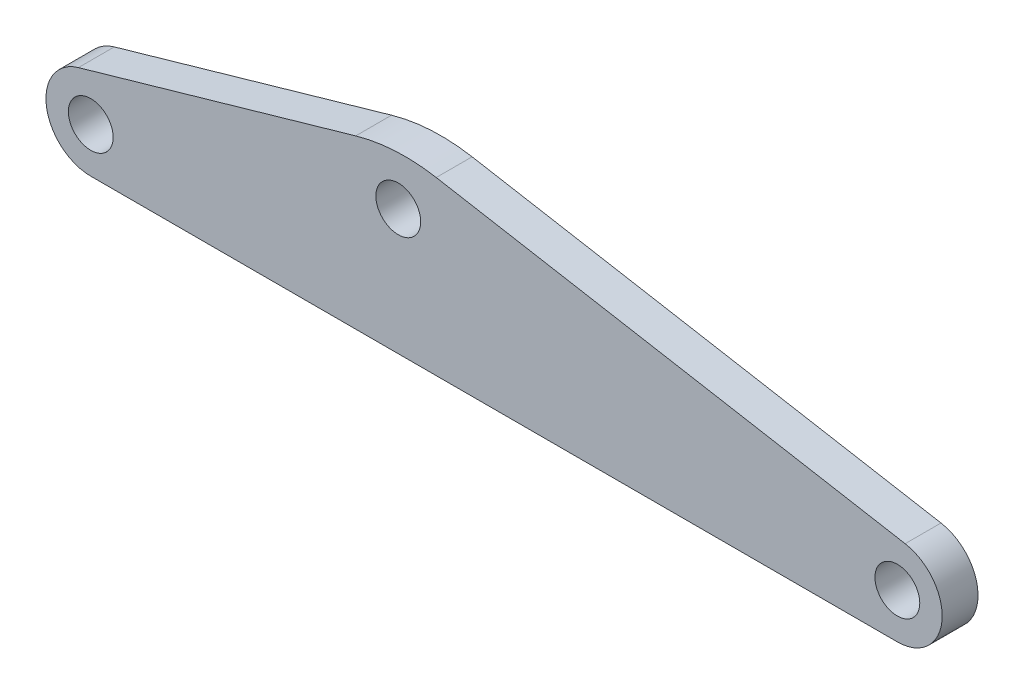
from build123d import *

# Parameters (mm, degrees)
LINK_PROFILE_SKETCH_R = 2.5
LINK_PLATE_4MM_DEPTH  = 4


with BuildPart() as part:
    # Link Profile Sketch → Link Plate 4mm (new body)
    with BuildSketch(Plane.XY):
        with BuildLine():
            Line((52.601773573, 0), (-37.398226427, 0))
            ThreePointArc((-37.398226427, 0), (-42.349566771, 4.304134495), (-38.776413207, 9.80630848))
            Line((-38.776413207, 9.80630848), (-7.835417757, 18.678496156))
            ThreePointArc((-7.835417757, 18.678496156), (-3.369389765, 19.425852932), (1.150292913, 19.149417297))
            Line((1.150292913, 19.149417297), (53.470014461, 9.924038765))
            ThreePointArc((53.470014461, 9.924038765), (57.582747063, 4.564221286), (52.601773573, 0))
        make_face()
        with Locations((-3.085032863, 14)):
            Circle(LINK_PROFILE_SKETCH_R, mode=Mode.SUBTRACT)
        with Locations((-37.398226427, 5)):
            Circle(LINK_PROFILE_SKETCH_R, mode=Mode.SUBTRACT)
        with Locations((52.601773573, 5)):
            Circle(LINK_PROFILE_SKETCH_R, mode=Mode.SUBTRACT)
    extrude(amount=LINK_PLATE_4MM_DEPTH)


solid = part.part
